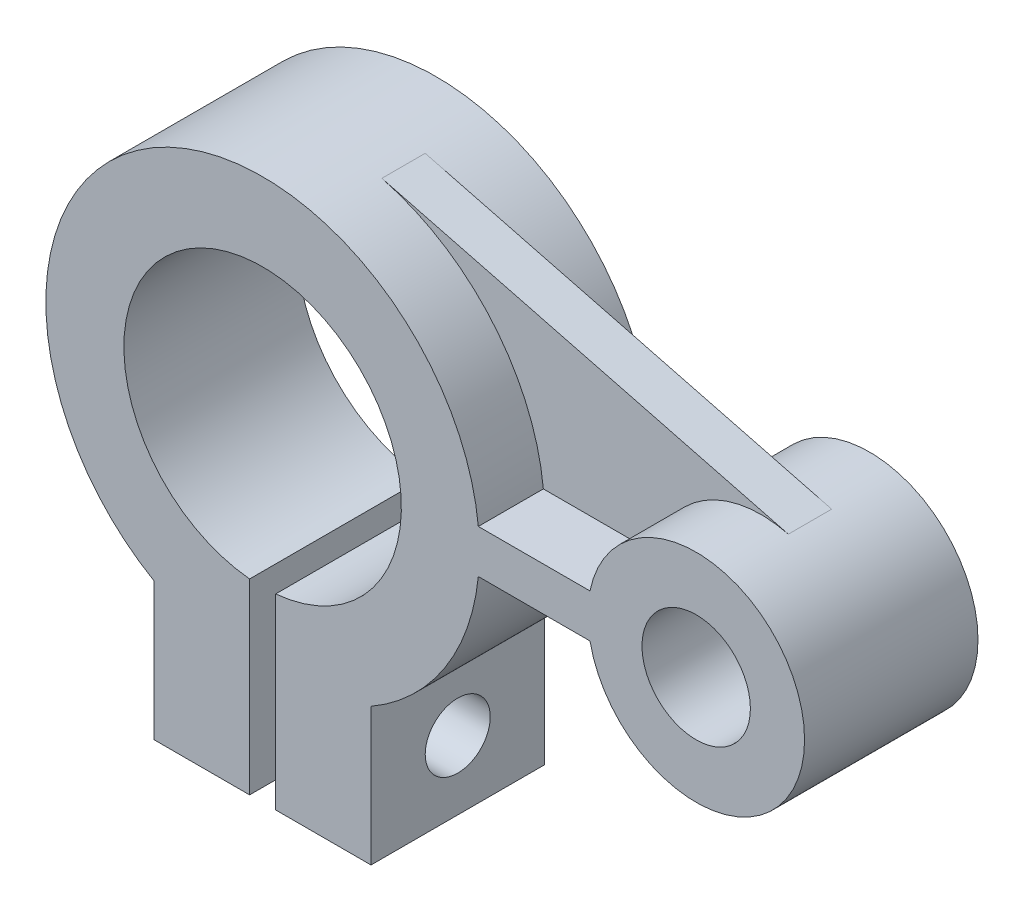
ISO-10303-21;
HEADER;
FILE_DESCRIPTION(('STEP AP214'),'2;1');
FILE_NAME('part.step','',(''),(''),'','','');
FILE_SCHEMA(('AUTOMOTIVE_DESIGN { 1 0 10303 214 1 1 1 1 }'));
ENDSEC;
DATA;
#1=APPLICATION_CONTEXT('core data for automotive mechanical design processes');
#2=APPLICATION_PROTOCOL_DEFINITION('international standard','automotive_design',2000,#1);
#3=PRODUCT_CONTEXT('',#1,'mechanical');
#4=PRODUCT('Part','Part','',(#3));
#5=PRODUCT_RELATED_PRODUCT_CATEGORY('part','',(#4));
#6=PRODUCT_DEFINITION_FORMATION('','',#4);
#7=PRODUCT_DEFINITION_CONTEXT('part definition',#1,'design');
#8=PRODUCT_DEFINITION('design','',#6,#7);
#9=PRODUCT_DEFINITION_SHAPE('','',#8);
#10=(LENGTH_UNIT() NAMED_UNIT(*) SI_UNIT(.MILLI.,.METRE.));
#11=(NAMED_UNIT(*) PLANE_ANGLE_UNIT() SI_UNIT($,.RADIAN.));
#12=(NAMED_UNIT(*) SI_UNIT($,.STERADIAN.) SOLID_ANGLE_UNIT());
#13=UNCERTAINTY_MEASURE_WITH_UNIT(LENGTH_MEASURE(1.E-05),#10,'distance_accuracy_value','');
#14=(GEOMETRIC_REPRESENTATION_CONTEXT(3) GLOBAL_UNCERTAINTY_ASSIGNED_CONTEXT((#13)) GLOBAL_UNIT_ASSIGNED_CONTEXT((#10,
#11,#12)) REPRESENTATION_CONTEXT('',''));
#15=CARTESIAN_POINT('',(0.,0.,0.));
#16=DIRECTION('',(0.,0.,1.));
#17=DIRECTION('',(1.,0.,0.));
#18=AXIS2_PLACEMENT_3D('',#15,#16,#17);
#19=CARTESIAN_POINT('',(32.,5.,20.));
#20=DIRECTION('',(0.,1.,0.));
#21=DIRECTION('',(0.,0.,1.));
#22=AXIS2_PLACEMENT_3D('',#19,#20,#21);
#23=PLANE('',#22);
#24=DIRECTION('',(0.,0.,-1.));
#25=VECTOR('',#24,1.);
#26=CARTESIAN_POINT('',(49.749371855331,5.,20.));
#27=LINE('',#26,#25);
#28=CARTESIAN_POINT('',(49.749371855331,5.,-20.));
#29=VERTEX_POINT('',#28);
#30=CARTESIAN_POINT('',(49.749371855331,5.,-5.));
#31=VERTEX_POINT('',#30);
#32=EDGE_CURVE('E48',#29,#31,#27,.F.);
#33=ORIENTED_EDGE('',*,*,#32,.T.);
#34=DIRECTION('',(1.,0.,0.));
#35=VECTOR('',#34,1.);
#36=CARTESIAN_POINT('',(32.,5.,-5.));
#37=LINE('',#36,#35);
#38=CARTESIAN_POINT('',(75.5051025721682,5.,-5.));
#39=VERTEX_POINT('',#38);
#40=EDGE_CURVE('E167',#31,#39,#37,.T.);
#41=ORIENTED_EDGE('',*,*,#40,.T.);
#42=DIRECTION('',(0.,0.,-1.));
#43=VECTOR('',#42,1.);
#44=CARTESIAN_POINT('',(75.5051025721682,5.,20.));
#45=LINE('',#44,#43);
#46=CARTESIAN_POINT('',(75.5051025721682,5.,-20.));
#47=VERTEX_POINT('',#46);
#48=EDGE_CURVE('E271',#47,#39,#45,.F.);
#49=ORIENTED_EDGE('',*,*,#48,.F.);
#50=DIRECTION('',(1.,0.,0.));
#51=VECTOR('',#50,1.);
#52=CARTESIAN_POINT('',(32.,5.,-20.));
#53=LINE('',#52,#51);
#54=EDGE_CURVE('E251',#29,#47,#53,.T.);
#55=ORIENTED_EDGE('',*,*,#54,.F.);
#56=EDGE_LOOP('',(#33,#41,#49,#55));
#57=FACE_BOUND('',#56,.T.);
#58=ADVANCED_FACE('F39',(#57),#23,.T.);
#59=CARTESIAN_POINT('',(32.,-5.,20.));
#60=DIRECTION('',(0.,1.,0.));
#61=DIRECTION('',(0.,0.,1.));
#62=AXIS2_PLACEMENT_3D('',#59,#60,#61);
#63=PLANE('',#62);
#64=DIRECTION('',(1.,0.,0.));
#65=VECTOR('',#64,1.);
#66=CARTESIAN_POINT('',(32.,-5.,20.));
#67=LINE('',#66,#65);
#68=CARTESIAN_POINT('',(49.749371855331,-5.,20.));
#69=VERTEX_POINT('',#68);
#70=CARTESIAN_POINT('',(75.5051025721682,-5.,20.));
#71=VERTEX_POINT('',#70);
#72=EDGE_CURVE('E248',#69,#71,#67,.T.);
#73=ORIENTED_EDGE('',*,*,#72,.F.);
#74=DIRECTION('',(0.,0.,-1.));
#75=VECTOR('',#74,1.);
#76=CARTESIAN_POINT('',(49.749371855331,-5.,20.));
#77=LINE('',#76,#75);
#78=CARTESIAN_POINT('',(49.749371855331,-5.,-20.));
#79=VERTEX_POINT('',#78);
#80=EDGE_CURVE('E242',#79,#69,#77,.F.);
#81=ORIENTED_EDGE('',*,*,#80,.F.);
#82=DIRECTION('',(1.,0.,0.));
#83=VECTOR('',#82,1.);
#84=CARTESIAN_POINT('',(32.,-5.,-20.));
#85=LINE('',#84,#83);
#86=CARTESIAN_POINT('',(75.5051025721682,-5.,-20.));
#87=VERTEX_POINT('',#86);
#88=EDGE_CURVE('E250',#79,#87,#85,.T.);
#89=ORIENTED_EDGE('',*,*,#88,.T.);
#90=DIRECTION('',(0.,0.,-1.));
#91=VECTOR('',#90,1.);
#92=CARTESIAN_POINT('',(75.5051025721682,-5.,20.));
#93=LINE('',#92,#91);
#94=EDGE_CURVE('E272',#87,#71,#93,.F.);
#95=ORIENTED_EDGE('',*,*,#94,.T.);
#96=EDGE_LOOP('',(#73,#81,#89,#95));
#97=FACE_BOUND('',#96,.T.);
#98=ADVANCED_FACE('F307',(#97),#63,.F.);
#99=DIRECTION('',(1.,0.,0.));
#100=VECTOR('',#99,1.);
#101=CARTESIAN_POINT('',(32.,5.,5.));
#102=LINE('',#101,#100);
#103=CARTESIAN_POINT('',(49.749371855331,5.,5.));
#104=VERTEX_POINT('',#103);
#105=CARTESIAN_POINT('',(75.5051025721682,5.,5.));
#106=VERTEX_POINT('',#105);
#107=EDGE_CURVE('E177',#104,#106,#102,.T.);
#108=ORIENTED_EDGE('',*,*,#107,.F.);
#109=CARTESIAN_POINT('',(49.749371855331,5.,20.));
#110=VERTEX_POINT('',#109);
#111=EDGE_CURVE('E274',#104,#110,#27,.F.);
#112=ORIENTED_EDGE('',*,*,#111,.T.);
#113=DIRECTION('',(1.,0.,0.));
#114=VECTOR('',#113,1.);
#115=CARTESIAN_POINT('',(32.,5.,20.));
#116=LINE('',#115,#114);
#117=CARTESIAN_POINT('',(75.5051025721682,5.,20.));
#118=VERTEX_POINT('',#117);
#119=EDGE_CURVE('E252',#110,#118,#116,.T.);
#120=ORIENTED_EDGE('',*,*,#119,.T.);
#121=EDGE_CURVE('E268',#106,#118,#45,.F.);
#122=ORIENTED_EDGE('',*,*,#121,.F.);
#123=EDGE_LOOP('',(#108,#112,#120,#122));
#124=FACE_BOUND('',#123,.T.);
#125=ADVANCED_FACE('F278',(#124),#23,.T.);
#126=CARTESIAN_POINT('',(100.,0.,20.));
#127=DIRECTION('',(0.,0.,-1.));
#128=DIRECTION('',(-1.,0.,0.));
#129=AXIS2_PLACEMENT_3D('',#126,#127,#128);
#130=CYLINDRICAL_SURFACE('',#129,25.);
#131=CARTESIAN_POINT('',(100.,0.,20.));
#132=DIRECTION('',(0.,0.,1.));
#133=DIRECTION('',(1.,0.,0.));
#134=AXIS2_PLACEMENT_3D('',#131,#132,#133);
#135=CIRCLE('',#134,25.);
#136=EDGE_CURVE('E264',#71,#118,#135,.T.);
#137=ORIENTED_EDGE('',*,*,#136,.F.);
#138=ORIENTED_EDGE('',*,*,#94,.F.);
#139=CARTESIAN_POINT('',(100.,0.,-20.));
#140=DIRECTION('',(0.,0.,1.));
#141=DIRECTION('',(1.,0.,0.));
#142=AXIS2_PLACEMENT_3D('',#139,#140,#141);
#143=CIRCLE('',#142,25.);
#144=EDGE_CURVE('E265',#87,#47,#143,.T.);
#145=ORIENTED_EDGE('',*,*,#144,.T.);
#146=ORIENTED_EDGE('',*,*,#48,.T.);
#147=CARTESIAN_POINT('',(100.,0.,-5.));
#148=DIRECTION('',(0.,0.,1.));
#149=DIRECTION('',(1.,0.,0.));
#150=AXIS2_PLACEMENT_3D('',#147,#148,#149);
#151=CIRCLE('',#150,25.);
#152=CARTESIAN_POINT('',(106.25,24.2061459137964,-5.));
#153=VERTEX_POINT('',#152);
#154=EDGE_CURVE('E58',#153,#39,#151,.T.);
#155=ORIENTED_EDGE('',*,*,#154,.F.);
#156=DIRECTION('',(0.,0.,-1.));
#157=VECTOR('',#156,1.);
#158=CARTESIAN_POINT('',(106.25,24.2061459137964,20.));
#159=LINE('',#158,#157);
#160=CARTESIAN_POINT('',(106.25,24.2061459137964,5.));
#161=VERTEX_POINT('',#160);
#162=EDGE_CURVE('E54',#161,#153,#159,.T.);
#163=ORIENTED_EDGE('',*,*,#162,.F.);
#164=CARTESIAN_POINT('',(100.,0.,5.));
#165=DIRECTION('',(0.,0.,1.));
#166=DIRECTION('',(1.,0.,0.));
#167=AXIS2_PLACEMENT_3D('',#164,#165,#166);
#168=CIRCLE('',#167,25.);
#169=EDGE_CURVE('E181',#161,#106,#168,.T.);
#170=ORIENTED_EDGE('',*,*,#169,.T.);
#171=ORIENTED_EDGE('',*,*,#121,.T.);
#172=EDGE_LOOP('',(#137,#138,#145,#146,#155,#163,#170,#171));
#173=FACE_BOUND('',#172,.T.);
#174=ADVANCED_FACE('F41',(#173),#130,.T.);
#175=CARTESIAN_POINT('',(100.,0.,20.));
#176=DIRECTION('',(0.,0.,1.));
#177=DIRECTION('',(1.,0.,0.));
#178=AXIS2_PLACEMENT_3D('',#175,#176,#177);
#179=PLANE('',#178);
#180=ORIENTED_EDGE('',*,*,#119,.F.);
#181=CARTESIAN_POINT('',(0.,0.,20.));
#182=DIRECTION('',(0.,0.,1.));
#183=DIRECTION('',(1.,0.,0.));
#184=AXIS2_PLACEMENT_3D('',#181,#182,#183);
#185=CIRCLE('',#184,50.);
#186=CARTESIAN_POINT('',(-25.,-43.3012701892219,20.));
#187=VERTEX_POINT('',#186);
#188=EDGE_CURVE('E245',#110,#187,#185,.T.);
#189=ORIENTED_EDGE('',*,*,#188,.T.);
#190=DIRECTION('',(0.,-1.,0.));
#191=VECTOR('',#190,1.);
#192=CARTESIAN_POINT('',(-25.,-43.3012701892219,20.));
#193=LINE('',#192,#191);
#194=CARTESIAN_POINT('',(-25.,-75.,20.));
#195=VERTEX_POINT('',#194);
#196=EDGE_CURVE('E218',#187,#195,#193,.T.);
#197=ORIENTED_EDGE('',*,*,#196,.T.);
#198=DIRECTION('',(1.,0.,0.));
#199=VECTOR('',#198,1.);
#200=CARTESIAN_POINT('',(-25.,-75.,20.));
#201=LINE('',#200,#199);
#202=CARTESIAN_POINT('',(-3.,-75.,20.));
#203=VERTEX_POINT('',#202);
#204=EDGE_CURVE('E226',#195,#203,#201,.T.);
#205=ORIENTED_EDGE('',*,*,#204,.T.);
#206=DIRECTION('',(0.,-1.,0.));
#207=VECTOR('',#206,1.);
#208=CARTESIAN_POINT('',(-3.00000000000001,-31.859064644148,20.));
#209=LINE('',#208,#207);
#210=CARTESIAN_POINT('',(-3.00000000000001,-31.859064644148,20.));
#211=VERTEX_POINT('',#210);
#212=EDGE_CURVE('E188',#211,#203,#209,.T.);
#213=ORIENTED_EDGE('',*,*,#212,.F.);
#214=CARTESIAN_POINT('',(0.,0.,20.));
#215=DIRECTION('',(0.,0.,1.));
#216=DIRECTION('',(1.,0.,0.));
#217=AXIS2_PLACEMENT_3D('',#214,#215,#216);
#218=CIRCLE('',#217,32.);
#219=CARTESIAN_POINT('',(2.99999999999998,-31.859064644148,20.));
#220=VERTEX_POINT('',#219);
#221=EDGE_CURVE('E232',#220,#211,#218,.T.);
#222=ORIENTED_EDGE('',*,*,#221,.F.);
#223=DIRECTION('',(0.,1.,0.));
#224=VECTOR('',#223,1.);
#225=CARTESIAN_POINT('',(3.00000000000001,-31.859064644148,20.));
#226=LINE('',#225,#224);
#227=CARTESIAN_POINT('',(3.,-75.,20.));
#228=VERTEX_POINT('',#227);
#229=EDGE_CURVE('E190',#228,#220,#226,.T.);
#230=ORIENTED_EDGE('',*,*,#229,.F.);
#231=CARTESIAN_POINT('',(25.,-75.,20.));
#232=VERTEX_POINT('',#231);
#233=EDGE_CURVE('E230',#228,#232,#201,.T.);
#234=ORIENTED_EDGE('',*,*,#233,.T.);
#235=DIRECTION('',(0.,1.,0.));
#236=VECTOR('',#235,1.);
#237=CARTESIAN_POINT('',(25.,-43.3012701892219,20.));
#238=LINE('',#237,#236);
#239=CARTESIAN_POINT('',(25.,-43.3012701892219,20.));
#240=VERTEX_POINT('',#239);
#241=EDGE_CURVE('E212',#232,#240,#238,.T.);
#242=ORIENTED_EDGE('',*,*,#241,.T.);
#243=EDGE_CURVE('E238',#240,#69,#185,.T.);
#244=ORIENTED_EDGE('',*,*,#243,.T.);
#245=ORIENTED_EDGE('',*,*,#72,.T.);
#246=ORIENTED_EDGE('',*,*,#136,.T.);
#247=EDGE_LOOP('',(#180,#189,#197,#205,#213,#222,#230,#234,#242,#244,#245,#246));
#248=FACE_BOUND('',#247,.T.);
#249=CARTESIAN_POINT('',(100.,0.,20.));
#250=DIRECTION('',(0.,0.,1.));
#251=DIRECTION('',(1.,0.,0.));
#252=AXIS2_PLACEMENT_3D('',#249,#250,#251);
#253=CIRCLE('',#252,12.5);
#254=CARTESIAN_POINT('',(112.5,0.,20.));
#255=VERTEX_POINT('',#254);
#256=EDGE_CURVE('E259',#255,#255,#253,.T.);
#257=ORIENTED_EDGE('',*,*,#256,.F.);
#258=EDGE_LOOP('',(#257));
#259=FACE_BOUND('',#258,.T.);
#260=ADVANCED_FACE('F286',(#248,#259),#179,.T.);
#261=CARTESIAN_POINT('',(100.,0.,-20.));
#262=DIRECTION('',(0.,0.,1.));
#263=DIRECTION('',(1.,0.,0.));
#264=AXIS2_PLACEMENT_3D('',#261,#262,#263);
#265=PLANE('',#264);
#266=ORIENTED_EDGE('',*,*,#88,.F.);
#267=CARTESIAN_POINT('',(0.,0.,-20.));
#268=DIRECTION('',(0.,0.,1.));
#269=DIRECTION('',(1.,0.,0.));
#270=AXIS2_PLACEMENT_3D('',#267,#268,#269);
#271=CIRCLE('',#270,50.);
#272=CARTESIAN_POINT('',(25.,-43.3012701892219,-20.));
#273=VERTEX_POINT('',#272);
#274=EDGE_CURVE('E241',#273,#79,#271,.T.);
#275=ORIENTED_EDGE('',*,*,#274,.F.);
#276=DIRECTION('',(0.,1.,0.));
#277=VECTOR('',#276,1.);
#278=CARTESIAN_POINT('',(25.,-43.3012701892219,-20.));
#279=LINE('',#278,#277);
#280=CARTESIAN_POINT('',(25.,-75.,-20.));
#281=VERTEX_POINT('',#280);
#282=EDGE_CURVE('E214',#281,#273,#279,.T.);
#283=ORIENTED_EDGE('',*,*,#282,.F.);
#284=DIRECTION('',(1.,0.,0.));
#285=VECTOR('',#284,1.);
#286=CARTESIAN_POINT('',(-25.,-75.,-20.));
#287=LINE('',#286,#285);
#288=CARTESIAN_POINT('',(3.,-75.,-20.));
#289=VERTEX_POINT('',#288);
#290=EDGE_CURVE('E217',#289,#281,#287,.T.);
#291=ORIENTED_EDGE('',*,*,#290,.F.);
#292=DIRECTION('',(0.,1.,0.));
#293=VECTOR('',#292,1.);
#294=CARTESIAN_POINT('',(3.00000000000001,-31.859064644148,-20.));
#295=LINE('',#294,#293);
#296=CARTESIAN_POINT('',(3.00000000000001,-31.859064644148,-20.));
#297=VERTEX_POINT('',#296);
#298=EDGE_CURVE('E192',#289,#297,#295,.T.);
#299=ORIENTED_EDGE('',*,*,#298,.T.);
#300=CARTESIAN_POINT('',(0.,0.,-20.));
#301=DIRECTION('',(0.,0.,1.));
#302=DIRECTION('',(1.,0.,0.));
#303=AXIS2_PLACEMENT_3D('',#300,#301,#302);
#304=CIRCLE('',#303,32.);
#305=CARTESIAN_POINT('',(-3.00000000000001,-31.859064644148,-20.));
#306=VERTEX_POINT('',#305);
#307=EDGE_CURVE('E228',#297,#306,#304,.T.);
#308=ORIENTED_EDGE('',*,*,#307,.T.);
#309=DIRECTION('',(0.,-1.,0.));
#310=VECTOR('',#309,1.);
#311=CARTESIAN_POINT('',(-3.00000000000001,-31.859064644148,-20.));
#312=LINE('',#311,#310);
#313=CARTESIAN_POINT('',(-3.,-75.,-20.));
#314=VERTEX_POINT('',#313);
#315=EDGE_CURVE('E191',#306,#314,#312,.T.);
#316=ORIENTED_EDGE('',*,*,#315,.T.);
#317=CARTESIAN_POINT('',(-25.,-75.,-20.));
#318=VERTEX_POINT('',#317);
#319=EDGE_CURVE('E219',#318,#314,#287,.T.);
#320=ORIENTED_EDGE('',*,*,#319,.F.);
#321=DIRECTION('',(0.,-1.,0.));
#322=VECTOR('',#321,1.);
#323=CARTESIAN_POINT('',(-25.,-43.3012701892219,-20.));
#324=LINE('',#323,#322);
#325=CARTESIAN_POINT('',(-25.,-43.3012701892219,-20.));
#326=VERTEX_POINT('',#325);
#327=EDGE_CURVE('E224',#326,#318,#324,.T.);
#328=ORIENTED_EDGE('',*,*,#327,.F.);
#329=EDGE_CURVE('E236',#29,#326,#271,.T.);
#330=ORIENTED_EDGE('',*,*,#329,.F.);
#331=ORIENTED_EDGE('',*,*,#54,.T.);
#332=ORIENTED_EDGE('',*,*,#144,.F.);
#333=EDGE_LOOP('',(#266,#275,#283,#291,#299,#308,#316,#320,#328,#330,#331,#332));
#334=FACE_BOUND('',#333,.T.);
#335=CARTESIAN_POINT('',(100.,0.,-20.));
#336=DIRECTION('',(0.,0.,1.));
#337=DIRECTION('',(1.,0.,0.));
#338=AXIS2_PLACEMENT_3D('',#335,#336,#337);
#339=CIRCLE('',#338,12.5);
#340=CARTESIAN_POINT('',(112.5,0.,-20.));
#341=VERTEX_POINT('',#340);
#342=EDGE_CURVE('E258',#341,#341,#339,.T.);
#343=ORIENTED_EDGE('',*,*,#342,.T.);
#344=EDGE_LOOP('',(#343));
#345=FACE_BOUND('',#344,.T.);
#346=ADVANCED_FACE('F322',(#334,#345),#265,.F.);
#347=CARTESIAN_POINT('',(100.,0.,20.));
#348=DIRECTION('',(0.,0.,-1.));
#349=DIRECTION('',(-1.,0.,0.));
#350=AXIS2_PLACEMENT_3D('',#347,#348,#349);
#351=CYLINDRICAL_SURFACE('',#350,12.5);
#352=ORIENTED_EDGE('',*,*,#256,.T.);
#353=EDGE_LOOP('',(#352));
#354=FACE_BOUND('',#353,.T.);
#355=ORIENTED_EDGE('',*,*,#342,.F.);
#356=EDGE_LOOP('',(#355));
#357=FACE_BOUND('',#356,.T.);
#358=ADVANCED_FACE('F327',(#354,#357),#351,.F.);
#359=CARTESIAN_POINT('',(0.,0.,20.));
#360=DIRECTION('',(0.,0.,-1.));
#361=DIRECTION('',(-1.,0.,0.));
#362=AXIS2_PLACEMENT_3D('',#359,#360,#361);
#363=CYLINDRICAL_SURFACE('',#362,50.);
#364=DIRECTION('',(0.,0.,-1.));
#365=VECTOR('',#364,1.);
#366=CARTESIAN_POINT('',(25.,-43.3012701892219,20.));
#367=LINE('',#366,#365);
#368=EDGE_CURVE('E209',#240,#273,#367,.T.);
#369=ORIENTED_EDGE('',*,*,#368,.T.);
#370=ORIENTED_EDGE('',*,*,#274,.T.);
#371=ORIENTED_EDGE('',*,*,#80,.T.);
#372=ORIENTED_EDGE('',*,*,#243,.F.);
#373=EDGE_LOOP('',(#369,#370,#371,#372));
#374=FACE_BOUND('',#373,.T.);
#375=ADVANCED_FACE('F332',(#374),#363,.T.);
#376=CARTESIAN_POINT('',(0.,0.,20.));
#377=DIRECTION('',(0.,0.,-1.));
#378=DIRECTION('',(-1.,0.,0.));
#379=AXIS2_PLACEMENT_3D('',#376,#377,#378);
#380=CYLINDRICAL_SURFACE('',#379,32.);
#381=ORIENTED_EDGE('',*,*,#221,.T.);
#382=DIRECTION('',(0.,0.,1.));
#383=VECTOR('',#382,1.);
#384=CARTESIAN_POINT('',(-3.00000000000001,-31.859064644148,-20.));
#385=LINE('',#384,#383);
#386=EDGE_CURVE('E200',#306,#211,#385,.T.);
#387=ORIENTED_EDGE('',*,*,#386,.F.);
#388=ORIENTED_EDGE('',*,*,#307,.F.);
#389=DIRECTION('',(0.,0.,1.));
#390=VECTOR('',#389,1.);
#391=CARTESIAN_POINT('',(3.00000000000001,-31.859064644148,-20.));
#392=LINE('',#391,#390);
#393=EDGE_CURVE('E205',#297,#220,#392,.T.);
#394=ORIENTED_EDGE('',*,*,#393,.T.);
#395=EDGE_LOOP('',(#381,#387,#388,#394));
#396=FACE_BOUND('',#395,.T.);
#397=ADVANCED_FACE('F338',(#396),#380,.F.);
#398=CARTESIAN_POINT('',(-25.,-75.,20.));
#399=DIRECTION('',(0.,1.,0.));
#400=DIRECTION('',(0.,0.,1.));
#401=AXIS2_PLACEMENT_3D('',#398,#399,#400);
#402=PLANE('',#401);
#403=ORIENTED_EDGE('',*,*,#233,.F.);
#404=DIRECTION('',(0.,0.,1.));
#405=VECTOR('',#404,1.);
#406=CARTESIAN_POINT('',(3.,-75.,-20.));
#407=LINE('',#406,#405);
#408=EDGE_CURVE('E204',#289,#228,#407,.T.);
#409=ORIENTED_EDGE('',*,*,#408,.F.);
#410=ORIENTED_EDGE('',*,*,#290,.T.);
#411=DIRECTION('',(0.,0.,-1.));
#412=VECTOR('',#411,1.);
#413=CARTESIAN_POINT('',(25.,-75.,20.));
#414=LINE('',#413,#412);
#415=EDGE_CURVE('E208',#232,#281,#414,.T.);
#416=ORIENTED_EDGE('',*,*,#415,.F.);
#417=EDGE_LOOP('',(#403,#409,#410,#416));
#418=FACE_BOUND('',#417,.T.);
#419=ADVANCED_FACE('F342',(#418),#402,.F.);
#420=CARTESIAN_POINT('',(0.,0.,5.));
#421=DIRECTION('',(0.,0.,1.));
#422=DIRECTION('',(1.,0.,0.));
#423=AXIS2_PLACEMENT_3D('',#420,#421,#422);
#424=CIRCLE('',#423,50.);
#425=CARTESIAN_POINT('',(12.5,48.4122918275927,5.));
#426=VERTEX_POINT('',#425);
#427=EDGE_CURVE('E156',#104,#426,#424,.T.);
#428=ORIENTED_EDGE('',*,*,#427,.T.);
#429=DIRECTION('',(0.,0.,-1.));
#430=VECTOR('',#429,1.);
#431=CARTESIAN_POINT('',(12.5,48.4122918275927,20.));
#432=LINE('',#431,#430);
#433=CARTESIAN_POINT('',(12.5,48.4122918275927,-5.));
#434=VERTEX_POINT('',#433);
#435=EDGE_CURVE('E11',#426,#434,#432,.T.);
#436=ORIENTED_EDGE('',*,*,#435,.T.);
#437=CARTESIAN_POINT('',(0.,0.,-5.));
#438=DIRECTION('',(0.,0.,1.));
#439=DIRECTION('',(1.,0.,0.));
#440=AXIS2_PLACEMENT_3D('',#437,#438,#439);
#441=CIRCLE('',#440,50.);
#442=EDGE_CURVE('E155',#31,#434,#441,.T.);
#443=ORIENTED_EDGE('',*,*,#442,.F.);
#444=ORIENTED_EDGE('',*,*,#32,.F.);
#445=ORIENTED_EDGE('',*,*,#329,.T.);
#446=DIRECTION('',(0.,0.,-1.));
#447=VECTOR('',#446,1.);
#448=CARTESIAN_POINT('',(-25.,-43.3012701892219,20.));
#449=LINE('',#448,#447);
#450=EDGE_CURVE('E215',#187,#326,#449,.T.);
#451=ORIENTED_EDGE('',*,*,#450,.F.);
#452=ORIENTED_EDGE('',*,*,#188,.F.);
#453=ORIENTED_EDGE('',*,*,#111,.F.);
#454=EDGE_LOOP('',(#428,#436,#443,#444,#445,#451,#452,#453));
#455=FACE_BOUND('',#454,.T.);
#456=ADVANCED_FACE('F151',(#455),#363,.T.);
#457=CARTESIAN_POINT('',(-25.,-43.3012701892219,20.));
#458=DIRECTION('',(1.,0.,0.));
#459=DIRECTION('',(0.,1.,0.));
#460=AXIS2_PLACEMENT_3D('',#457,#458,#459);
#461=PLANE('',#460);
#462=CARTESIAN_POINT('',(-25.,-59.150635094611,0.));
#463=DIRECTION('',(1.,0.,0.));
#464=DIRECTION('',(0.,1.,0.));
#465=AXIS2_PLACEMENT_3D('',#462,#463,#464);
#466=CIRCLE('',#465,7.5);
#467=CARTESIAN_POINT('',(-25.,-51.650635094611,0.));
#468=VERTEX_POINT('',#467);
#469=EDGE_CURVE('E168',#468,#468,#466,.T.);
#470=ORIENTED_EDGE('',*,*,#469,.T.);
#471=EDGE_LOOP('',(#470));
#472=FACE_BOUND('',#471,.T.);
#473=ORIENTED_EDGE('',*,*,#450,.T.);
#474=ORIENTED_EDGE('',*,*,#327,.T.);
#475=DIRECTION('',(0.,0.,-1.));
#476=VECTOR('',#475,1.);
#477=CARTESIAN_POINT('',(-25.,-75.,20.));
#478=LINE('',#477,#476);
#479=EDGE_CURVE('E203',#195,#318,#478,.T.);
#480=ORIENTED_EDGE('',*,*,#479,.F.);
#481=ORIENTED_EDGE('',*,*,#196,.F.);
#482=EDGE_LOOP('',(#473,#474,#480,#481));
#483=FACE_BOUND('',#482,.T.);
#484=ADVANCED_FACE('F349',(#472,#483),#461,.F.);
#485=ORIENTED_EDGE('',*,*,#479,.T.);
#486=ORIENTED_EDGE('',*,*,#319,.T.);
#487=DIRECTION('',(0.,0.,1.));
#488=VECTOR('',#487,1.);
#489=CARTESIAN_POINT('',(-3.,-75.,-20.));
#490=LINE('',#489,#488);
#491=EDGE_CURVE('E196',#314,#203,#490,.T.);
#492=ORIENTED_EDGE('',*,*,#491,.T.);
#493=ORIENTED_EDGE('',*,*,#204,.F.);
#494=EDGE_LOOP('',(#485,#486,#492,#493));
#495=FACE_BOUND('',#494,.T.);
#496=ADVANCED_FACE('F351',(#495),#402,.F.);
#497=CARTESIAN_POINT('',(25.,-43.3012701892219,20.));
#498=DIRECTION('',(-1.,0.,0.));
#499=DIRECTION('',(0.,-1.,0.));
#500=AXIS2_PLACEMENT_3D('',#497,#498,#499);
#501=PLANE('',#500);
#502=CARTESIAN_POINT('',(25.,-59.150635094611,0.));
#503=DIRECTION('',(-1.,0.,0.));
#504=DIRECTION('',(0.,-1.,0.));
#505=AXIS2_PLACEMENT_3D('',#502,#503,#504);
#506=CIRCLE('',#505,7.5);
#507=CARTESIAN_POINT('',(25.,-66.650635094611,0.));
#508=VERTEX_POINT('',#507);
#509=EDGE_CURVE('E175',#508,#508,#506,.T.);
#510=ORIENTED_EDGE('',*,*,#509,.T.);
#511=EDGE_LOOP('',(#510));
#512=FACE_BOUND('',#511,.T.);
#513=ORIENTED_EDGE('',*,*,#415,.T.);
#514=ORIENTED_EDGE('',*,*,#282,.T.);
#515=ORIENTED_EDGE('',*,*,#368,.F.);
#516=ORIENTED_EDGE('',*,*,#241,.F.);
#517=EDGE_LOOP('',(#513,#514,#515,#516));
#518=FACE_BOUND('',#517,.T.);
#519=ADVANCED_FACE('F365',(#512,#518),#501,.F.);
#520=CARTESIAN_POINT('',(3.00000000000001,-31.859064644148,-20.));
#521=DIRECTION('',(1.,0.,0.));
#522=DIRECTION('',(0.,1.,0.));
#523=AXIS2_PLACEMENT_3D('',#520,#521,#522);
#524=PLANE('',#523);
#525=CARTESIAN_POINT('',(3.,-59.150635094611,0.));
#526=DIRECTION('',(1.,0.,0.));
#527=DIRECTION('',(0.,1.,0.));
#528=AXIS2_PLACEMENT_3D('',#525,#526,#527);
#529=CIRCLE('',#528,7.5);
#530=CARTESIAN_POINT('',(3.,-51.650635094611,0.));
#531=VERTEX_POINT('',#530);
#532=EDGE_CURVE('E407',#531,#531,#529,.T.);
#533=ORIENTED_EDGE('',*,*,#532,.T.);
#534=EDGE_LOOP('',(#533));
#535=FACE_BOUND('',#534,.T.);
#536=ORIENTED_EDGE('',*,*,#229,.T.);
#537=ORIENTED_EDGE('',*,*,#393,.F.);
#538=ORIENTED_EDGE('',*,*,#298,.F.);
#539=ORIENTED_EDGE('',*,*,#408,.T.);
#540=EDGE_LOOP('',(#536,#537,#538,#539));
#541=FACE_BOUND('',#540,.T.);
#542=ADVANCED_FACE('F369',(#535,#541),#524,.F.);
#543=CARTESIAN_POINT('',(-3.00000000000001,-31.859064644148,-20.));
#544=DIRECTION('',(-1.,0.,0.));
#545=DIRECTION('',(0.,-1.,0.));
#546=AXIS2_PLACEMENT_3D('',#543,#544,#545);
#547=PLANE('',#546);
#548=CARTESIAN_POINT('',(-3.,-59.150635094611,0.));
#549=DIRECTION('',(-1.,0.,0.));
#550=DIRECTION('',(0.,-1.,0.));
#551=AXIS2_PLACEMENT_3D('',#548,#549,#550);
#552=CIRCLE('',#551,7.5);
#553=CARTESIAN_POINT('',(-3.,-66.650635094611,0.));
#554=VERTEX_POINT('',#553);
#555=EDGE_CURVE('E43',#554,#554,#552,.T.);
#556=ORIENTED_EDGE('',*,*,#555,.T.);
#557=EDGE_LOOP('',(#556));
#558=FACE_BOUND('',#557,.T.);
#559=ORIENTED_EDGE('',*,*,#212,.T.);
#560=ORIENTED_EDGE('',*,*,#491,.F.);
#561=ORIENTED_EDGE('',*,*,#315,.F.);
#562=ORIENTED_EDGE('',*,*,#386,.T.);
#563=EDGE_LOOP('',(#559,#560,#561,#562));
#564=FACE_BOUND('',#563,.T.);
#565=ADVANCED_FACE('F305',(#558,#564),#547,.F.);
#566=CARTESIAN_POINT('',(106.25,24.2061459137964,0.));
#567=DIRECTION('',(0.25,0.968245836551854,0.));
#568=DIRECTION('',(-0.968245836551854,0.25,0.));
#569=AXIS2_PLACEMENT_3D('',#566,#567,#568);
#570=PLANE('',#569);
#571=DIRECTION('',(-0.968245836551854,0.25,0.));
#572=VECTOR('',#571,1.);
#573=CARTESIAN_POINT('',(106.25,24.2061459137964,5.));
#574=LINE('',#573,#572);
#575=EDGE_CURVE('E170',#161,#426,#574,.T.);
#576=ORIENTED_EDGE('',*,*,#575,.F.);
#577=ORIENTED_EDGE('',*,*,#162,.T.);
#578=DIRECTION('',(-0.968245836551854,0.25,0.));
#579=VECTOR('',#578,1.);
#580=CARTESIAN_POINT('',(106.25,24.2061459137964,-5.));
#581=LINE('',#580,#579);
#582=EDGE_CURVE('E164',#153,#434,#581,.T.);
#583=ORIENTED_EDGE('',*,*,#582,.T.);
#584=ORIENTED_EDGE('',*,*,#435,.F.);
#585=EDGE_LOOP('',(#576,#577,#583,#584));
#586=FACE_BOUND('',#585,.T.);
#587=ADVANCED_FACE('F166',(#586),#570,.T.);
#588=CARTESIAN_POINT('',(37.5,-12.5,5.));
#589=DIRECTION('',(0.,0.,1.));
#590=DIRECTION('',(1.,0.,0.));
#591=AXIS2_PLACEMENT_3D('',#588,#589,#590);
#592=PLANE('',#591);
#593=ORIENTED_EDGE('',*,*,#169,.F.);
#594=ORIENTED_EDGE('',*,*,#575,.T.);
#595=ORIENTED_EDGE('',*,*,#427,.F.);
#596=ORIENTED_EDGE('',*,*,#107,.T.);
#597=EDGE_LOOP('',(#593,#594,#595,#596));
#598=FACE_BOUND('',#597,.T.);
#599=ADVANCED_FACE('F294',(#598),#592,.T.);
#600=CARTESIAN_POINT('',(37.5,-12.5,-5.));
#601=DIRECTION('',(0.,0.,1.));
#602=DIRECTION('',(1.,0.,0.));
#603=AXIS2_PLACEMENT_3D('',#600,#601,#602);
#604=PLANE('',#603);
#605=ORIENTED_EDGE('',*,*,#582,.F.);
#606=ORIENTED_EDGE('',*,*,#154,.T.);
#607=ORIENTED_EDGE('',*,*,#40,.F.);
#608=ORIENTED_EDGE('',*,*,#442,.T.);
#609=EDGE_LOOP('',(#605,#606,#607,#608));
#610=FACE_BOUND('',#609,.T.);
#611=ADVANCED_FACE('F163',(#610),#604,.F.);
#612=CARTESIAN_POINT('',(-50.,-59.150635094611,0.));
#613=DIRECTION('',(1.,0.,0.));
#614=DIRECTION('',(0.,0.,-1.));
#615=AXIS2_PLACEMENT_3D('',#612,#613,#614);
#616=CYLINDRICAL_SURFACE('',#615,7.5);
#617=ORIENTED_EDGE('',*,*,#555,.F.);
#618=EDGE_LOOP('',(#617));
#619=FACE_BOUND('',#618,.T.);
#620=ORIENTED_EDGE('',*,*,#469,.F.);
#621=EDGE_LOOP('',(#620));
#622=FACE_BOUND('',#621,.T.);
#623=ADVANCED_FACE('F304',(#619,#622),#616,.F.);
#624=ORIENTED_EDGE('',*,*,#532,.F.);
#625=EDGE_LOOP('',(#624));
#626=FACE_BOUND('',#625,.T.);
#627=ORIENTED_EDGE('',*,*,#509,.F.);
#628=EDGE_LOOP('',(#627));
#629=FACE_BOUND('',#628,.T.);
#630=ADVANCED_FACE('F418',(#626,#629),#616,.F.);
#631=CLOSED_SHELL('',(#58,#98,#125,#174,#260,#346,#358,#375,#397,#419,#456,#484,#496,#519,#542,
#565,#587,#599,#611,#623,#630));
#632=MANIFOLD_SOLID_BREP('B2',#631);
#633=ADVANCED_BREP_SHAPE_REPRESENTATION('',(#18,#632),#14);
#634=SHAPE_DEFINITION_REPRESENTATION(#9,#633);
ENDSEC;
END-ISO-10303-21;
